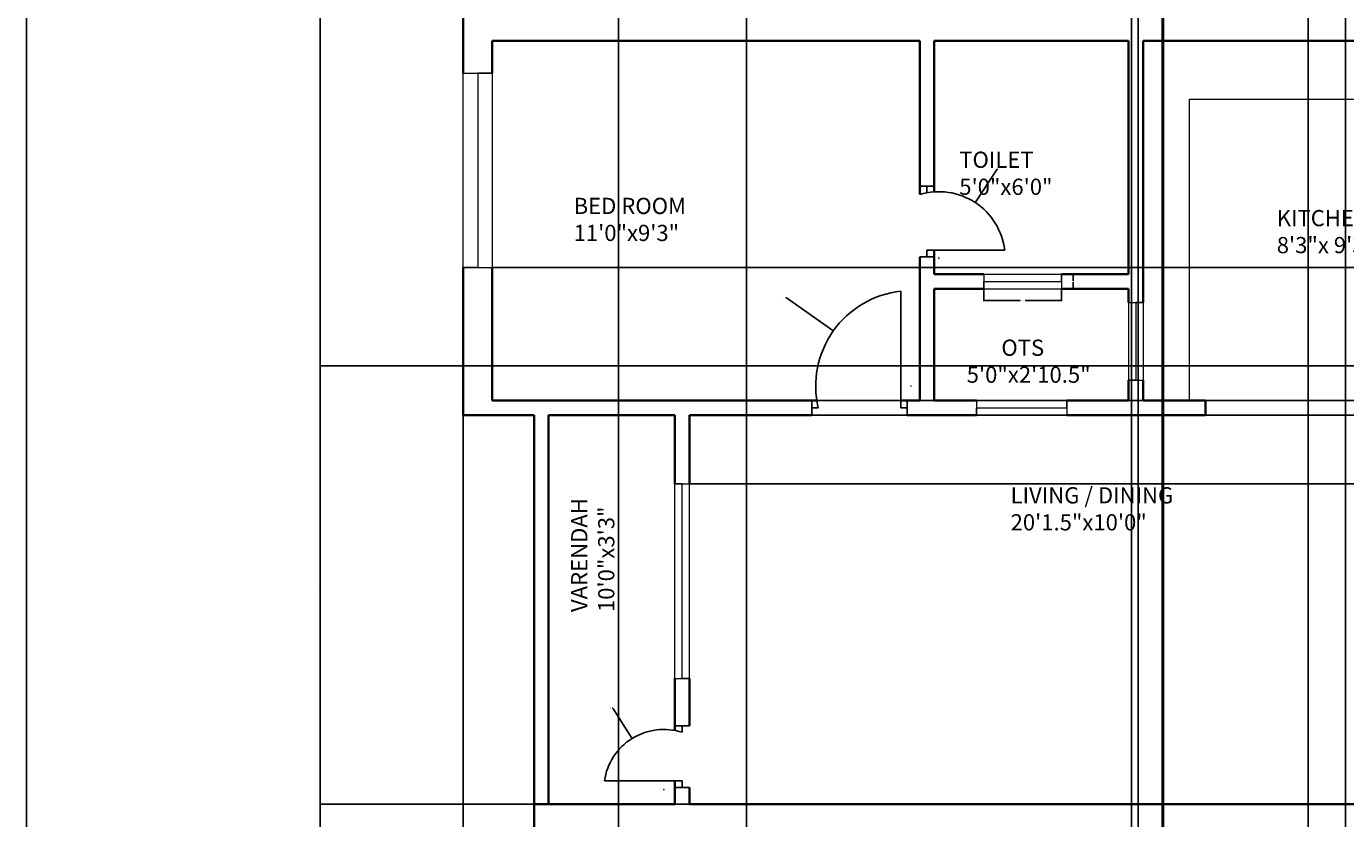
# Model space of a CAD drawing. Units: inches. Extents: x 1870 to 2611, y 1432 to 2511.
# Tile 3 of 5: x 1870 to 2277, y 1903 to 2147. Entities that reach past the tile are written whole.
import ezdxf

# ---------------------------------------------------------------- set-up
doc = ezdxf.new("R2010")
doc.units = ezdxf.units.IN
for name, color, linetype, lineweight in [('A-ANNO-DIMS', 2, 'Continuous', 18), ('A-ANNO-TTLB', 7, 'Continuous', 25), ('A-AREA-IDEN', 7, 'Continuous', 18), ('A-DOOR', 31, 'Continuous', 25), ('A-FLOR-FIXT', 8, 'Continuous', 18), ('A-GLAZ', 201, 'Continuous', 18), ('A-WALL', 7, 'Continuous', 35)]:
    doc.layers.add(name, color=color, linetype=linetype, lineweight=lineweight)
doc.styles.get("Standard").update_dxf_attribs({"font": 'arial.ttf'})
doc.dimstyles.get("Standard").update_dxf_attribs({"dimtxt": 0.18, "dimasz": 0.18, "dimexe": 0.18, "dimexo": 0.0625, "dimgap": 0.09, "dimtad": 0, "dimtih": 1, "dimtoh": 1, "dimdec": 4, "dimzin": 0, "dimdsep": 46, "dimtxsty": 'Standard', "dimcen": 0.09, "dimadec": 0, "dimazin": 0, "dimtfac": 1, "dimtdec": 4, "dimtofl": 0, "dimtmove": 0, "dimatfit": 3, "dimfxl": 1, "dimtolj": 1, "dimtzin": 0, "dimarcsym": 0})

# ---------------------------------------------------------------- blocks, each defined once
blk = doc.blocks.new('DOOR-LEAF-36-JAMB-4P5')
for p, q in [((36, 2), (0, 2)), ((33.75, 0), (38.25, 0)), ((36, 0), (36, 2)), ((38.25, 0), (36, 0))]:
    blk.add_line(p, q)
blk = doc.blocks.new('DOOR-LEAF-24-JAMB-4P5')
for p, q in [((2, 2.25), (2, 26.25)), ((0, 4.5), (0, 0)), ((0, 0), (0, 2.25)), ((0, 2.25), (2, 2.25))]:
    blk.add_line(p, q)
blk = doc.blocks.new('WIN-60-FRAME-9')
for p, q in [((0, 9), (0, 0)), ((60, 9), (0, 9)), ((60, 4.5), (60, 9)), ((60, 9), (60, 0)), ((0, 0), (0, 4.5)), ((0, 4.5), (60, 4.5)), ((0, 0), (60, 0))]:
    blk.add_line(p, q)
blk = doc.blocks.new('WIN-24-FRAME-4P5')
for p, q in [((0, 4.5), (0, 0)), ((0, 4.5), (24, 4.5)), ((24, 2.25), (24, 4.5)), ((24, 4.5), (24, 0)), ((0, 0), (0, 2.25)), ((0, 2.25), (24, 2.25)), ((0, 0), (24, 0))]:
    blk.add_line(p, q)
blk = doc.blocks.new('WIN-60-FRAME-4P5')
for p, q in [((0, 60), (4.5, 60)), ((0, 60), (0, 0)), ((4.5, 60), (2.25, 60)), ((2.25, 60), (2.25, 0)), ((4.5, 60), (4.5, 0)), ((2.25, 0), (0, 0)), ((0, 0), (4.5, 0))]:
    blk.add_line(p, q)
blk = doc.blocks.new('*D23')
at = {"layer": 'A-ANNO-DIMS', "color": 0, "lineweight": -2, "transparency": 16777216}
for p, q in [((2165.45, 2066.3), (2165.45, 2062.59)), ((2189.45, 2066.3), (2189.45, 2062.59)), ((2165.63, 2062.77), (2176.7, 2062.77)), ((2189.27, 2062.77), (2178.21, 2062.77))]:
    blk.add_line(p, q, dxfattribs=at)
at = {"layer": 'A-ANNO-DIMS', "color": 0, "transparency": 16777216}
for points in [[(2165.63, 2062.8), (2165.63, 2062.74), (2165.45, 2062.77)], [(2189.27, 2062.8), (2189.27, 2062.74), (2189.45, 2062.77)]]:
    blk.add_solid(points, dxfattribs=at)
at = {"layer": 'Defpoints', "color": 0, "transparency": 16777216}
for p in [(2165.45, 2066.37), (2189.45, 2066.37), (2189.45, 2062.77)]:
    blk.add_point(p, dxfattribs=at)
at = {"layer": 'A-ANNO-DIMS', "color": 0, "transparency": 16777216, "insert": (2177.45, 2062.77), "char_height": 0.18, "attachment_point": 5}
blk.add_mtext('\\A1;W4 24 TYP.', dxfattribs=at)
blk = doc.blocks.new('*D24')
at = {"layer": 'A-ANNO-DIMS', "color": 0, "lineweight": -2, "transparency": 16777216}
for p, q in [((2189.51, 2070.87), (2193.23, 2070.87)), ((2193.05, 2070.69), (2193.05, 2068.8)), ((2189.51, 2066.37), (2193.23, 2066.37)), ((2193.05, 2066.55), (2193.05, 2068.44))]:
    blk.add_line(p, q, dxfattribs=at)
at = {"layer": 'A-ANNO-DIMS', "color": 0, "transparency": 16777216}
for points in [[(2193.02, 2070.69), (2193.08, 2070.69), (2193.05, 2070.87)], [(2193.02, 2066.55), (2193.08, 2066.55), (2193.05, 2066.37)]]:
    blk.add_solid(points, dxfattribs=at)
at = {"layer": 'Defpoints', "color": 0, "transparency": 16777216}
for p in [(2189.45, 2070.87), (2193.05, 2070.87), (2189.45, 2066.37)]:
    blk.add_point(p, dxfattribs=at)
at = {"layer": 'A-ANNO-DIMS', "color": 0, "transparency": 16777216, "insert": (2193.05, 2068.62), "char_height": 0.18, "attachment_point": 5}
blk.add_mtext('\\A1;5 TYP.', dxfattribs=at)
blk = doc.blocks.new('*D28')
at = {"layer": 'A-ANNO-DIMS', "color": 0, "lineweight": -2, "transparency": 16777216}
for p, q in [((2004.57, 2151.87), (1960.31, 2151.87)), ((1960.49, 2151.69), (1960.49, 2029.8)), ((1960.49, 1907.55), (1960.49, 2029.44)), ((2026.46, 1907.37), (1960.31, 1907.37))]:
    blk.add_line(p, q, dxfattribs=at)
at = {"layer": 'A-ANNO-DIMS', "color": 0, "transparency": 16777216}
for points in [[(1960.46, 2151.69), (1960.52, 2151.69), (1960.49, 2151.87)], [(1960.46, 1907.55), (1960.52, 1907.55), (1960.49, 1907.37)]]:
    blk.add_solid(points, dxfattribs=at)
at = {"layer": 'Defpoints', "color": 0, "transparency": 16777216}
for p in [(2004.64, 2151.87), (1960.49, 1907.37), (2026.52, 1907.37)]:
    blk.add_point(p, dxfattribs=at)
at = {"layer": 'A-ANNO-DIMS', "color": 0, "transparency": 16777216, "insert": (1960.49, 2029.62), "char_height": 0.18, "attachment_point": 5}
blk.add_mtext('\\A1;244.5', dxfattribs=at)
blk = doc.blocks.new('*D29')
at = {"layer": 'A-ANNO-DIMS', "color": 0, "lineweight": -2, "transparency": 16777216}
for p, q in [((2026.46, 1907.37), (1960.31, 1907.37)), ((1960.49, 1907.19), (1960.49, 1774.05)), ((1960.49, 1640.55), (1960.49, 1773.69)), ((2026.46, 1640.37), (1960.31, 1640.37))]:
    blk.add_line(p, q, dxfattribs=at)
at = {"layer": 'A-ANNO-DIMS', "color": 0, "transparency": 16777216}
for points in [[(1960.46, 1907.19), (1960.52, 1907.19), (1960.49, 1907.37)], [(1960.46, 1640.55), (1960.52, 1640.55), (1960.49, 1640.37)]]:
    blk.add_solid(points, dxfattribs=at)
at = {"layer": 'Defpoints', "color": 0, "transparency": 16777216}
for p in [(2026.52, 1907.37), (1960.49, 1640.37), (2026.52, 1640.37)]:
    blk.add_point(p, dxfattribs=at)
at = {"layer": 'A-ANNO-DIMS', "color": 0, "transparency": 16777216, "insert": (1960.49, 1773.87), "char_height": 0.18, "attachment_point": 5}
blk.add_mtext('\\A1;267', dxfattribs=at)
blk = doc.blocks.new('*D30')
at = {"layer": 'A-ANNO-DIMS', "color": 0, "lineweight": -2, "transparency": 16777216}
for p, q in [((2004.64, 2027.3), (2004.64, 1485.35)), ((2026.52, 2027.3), (2026.52, 1485.35)), ((2004.82, 1485.53), (2015.11, 1485.53)), ((2026.34, 1485.53), (2016.04, 1485.53))]:
    blk.add_line(p, q, dxfattribs=at)
at = {"layer": 'A-ANNO-DIMS', "color": 0, "transparency": 16777216}
for points in [[(2004.82, 1485.56), (2004.82, 1485.5), (2004.64, 1485.53)], [(2026.34, 1485.56), (2026.34, 1485.5), (2026.52, 1485.53)]]:
    blk.add_solid(points, dxfattribs=at)
at = {"layer": 'Defpoints', "color": 0, "transparency": 16777216}
for p in [(2004.64, 2027.37), (2026.52, 2027.37), (2026.52, 1485.53)]:
    blk.add_point(p, dxfattribs=at)
at = {"layer": 'A-ANNO-DIMS', "color": 0, "transparency": 16777216, "insert": (2015.58, 1485.53), "char_height": 0.18, "attachment_point": 5}
blk.add_mtext('\\A1;21.882', dxfattribs=at)
blk = doc.blocks.new('*D34')
at = {"layer": 'A-ANNO-DIMS', "color": 0, "lineweight": -2, "transparency": 16777216}
for p, q in [((2385.57, 2042.61), (1960.31, 2042.61)), ((1960.49, 2042.43), (1960.49, 1975.17)), ((1960.49, 1907.55), (1960.49, 1974.8)), ((2385.57, 1907.37), (1960.31, 1907.37))]:
    blk.add_line(p, q, dxfattribs=at)
at = {"layer": 'A-ANNO-DIMS', "color": 0, "transparency": 16777216}
for points in [[(1960.46, 2042.43), (1960.52, 2042.43), (1960.49, 2042.61)], [(1960.46, 1907.55), (1960.52, 1907.55), (1960.49, 1907.37)]]:
    blk.add_solid(points, dxfattribs=at)
at = {"layer": 'Defpoints', "color": 0, "transparency": 16777216}
for p in [(1960.49, 2042.61), (2385.64, 2042.61), (2385.64, 1907.37)]:
    blk.add_point(p, dxfattribs=at)
at = {"layer": 'A-ANNO-DIMS', "color": 0, "transparency": 16777216, "insert": (1960.49, 1974.99), "char_height": 0.18, "attachment_point": 5}
blk.add_mtext('\\A1;135.24', dxfattribs=at)
blk = doc.blocks.new('*D39')
at = {"layer": 'A-ANNO-DIMS', "color": 0, "lineweight": -2, "transparency": 16777216}
for p, q in [((2052.64, 2396.3), (2052.64, 1485.35)), ((2092.09, 2396.3), (2092.09, 1485.35)), ((2052.82, 1485.53), (2071.97, 1485.53)), ((2091.91, 1485.53), (2072.76, 1485.53))]:
    blk.add_line(p, q, dxfattribs=at)
at = {"layer": 'A-ANNO-DIMS', "color": 0, "transparency": 16777216}
for points in [[(2052.82, 1485.56), (2052.82, 1485.5), (2052.64, 1485.53)], [(2091.91, 1485.56), (2091.91, 1485.5), (2092.09, 1485.53)]]:
    blk.add_solid(points, dxfattribs=at)
at = {"layer": 'Defpoints', "color": 0, "transparency": 16777216}
for p in [(2052.64, 2396.37), (2092.09, 2396.37), (2092.09, 1485.53)]:
    blk.add_point(p, dxfattribs=at)
at = {"layer": 'A-ANNO-DIMS', "color": 0, "transparency": 16777216, "insert": (2072.36, 1485.53), "char_height": 0.18, "attachment_point": 5}
blk.add_mtext('\\A1;39.45', dxfattribs=at)
blk = doc.blocks.new('*D40')
at = {"layer": 'A-ANNO-DIMS', "color": 0, "lineweight": -2, "transparency": 16777216}
for p, q in [((2213.14, 2396.3), (2213.14, 1485.35)), ((2220.9, 2396.3), (2220.9, 1485.35)), ((2213.32, 1485.53), (2216.63, 1485.53)), ((2220.72, 1485.53), (2217.41, 1485.53))]:
    blk.add_line(p, q, dxfattribs=at)
at = {"layer": 'A-ANNO-DIMS', "color": 0, "transparency": 16777216}
for points in [[(2213.32, 1485.56), (2213.32, 1485.5), (2213.14, 1485.53)], [(2220.72, 1485.56), (2220.72, 1485.5), (2220.9, 1485.53)]]:
    blk.add_solid(points, dxfattribs=at)
at = {"layer": 'Defpoints', "color": 0, "transparency": 16777216}
for p in [(2213.14, 2396.37), (2220.9, 2396.37), (2220.9, 1485.53)]:
    blk.add_point(p, dxfattribs=at)
at = {"layer": 'A-ANNO-DIMS', "color": 0, "transparency": 16777216, "insert": (2217.02, 1485.53), "char_height": 0.18, "attachment_point": 5}
blk.add_mtext('\\A1;7.766', dxfattribs=at)
blk = doc.blocks.new('*D41')
at = {"layer": 'A-ANNO-DIMS', "color": 0, "lineweight": -2, "transparency": 16777216}
for p, q in [((2265.64, 2396.3), (2265.64, 1485.35)), ((2277.17, 2396.3), (2277.17, 1485.35)), ((2265.82, 1485.53), (2270.95, 1485.53)), ((2276.99, 1485.53), (2271.86, 1485.53))]:
    blk.add_line(p, q, dxfattribs=at)
at = {"layer": 'A-ANNO-DIMS', "color": 0, "transparency": 16777216}
for points in [[(2265.82, 1485.56), (2265.82, 1485.5), (2265.64, 1485.53)], [(2276.99, 1485.56), (2276.99, 1485.5), (2277.17, 1485.53)]]:
    blk.add_solid(points, dxfattribs=at)
at = {"layer": 'Defpoints', "color": 0, "transparency": 16777216}
for p in [(2265.64, 2396.37), (2277.17, 2396.37), (2277.17, 1485.53)]:
    blk.add_point(p, dxfattribs=at)
at = {"layer": 'A-ANNO-DIMS', "color": 0, "transparency": 16777216, "insert": (2271.4, 1485.53), "char_height": 0.18, "attachment_point": 5}
blk.add_mtext('\\A1;11.535', dxfattribs=at)
blk = doc.blocks.new('*D45')
at = {"layer": 'A-ANNO-DIMS', "color": 0, "lineweight": -2, "transparency": 16777216}
for p, q in [((2211.02, 1649.43), (2211.02, 2449.7)), ((2211.2, 2449.52), (2215.39, 2449.52)), ((2220.38, 2449.52), (2216.18, 2449.52)), ((2220.56, 1649.43), (2220.56, 2449.7))]:
    blk.add_line(p, q, dxfattribs=at)
at = {"layer": 'A-ANNO-DIMS', "color": 0, "transparency": 16777216}
for points in [[(2211.2, 2449.55), (2211.2, 2449.49), (2211.02, 2449.52)], [(2220.38, 2449.55), (2220.38, 2449.49), (2220.56, 2449.52)]]:
    blk.add_solid(points, dxfattribs=at)
at = {"layer": 'Defpoints', "color": 0, "transparency": 16777216}
for p in [(2220.56, 2449.52), (2211.02, 1649.37), (2220.56, 1649.37)]:
    blk.add_point(p, dxfattribs=at)
at = {"layer": 'A-ANNO-DIMS', "color": 0, "transparency": 16777216, "insert": (2215.79, 2449.52), "char_height": 0.18, "attachment_point": 5}
blk.add_mtext('\\A1;9.537', dxfattribs=at)
blk = doc.blocks.new('*D51')
at = {"layer": 'A-ANNO-DIMS', "color": 0, "lineweight": -2, "transparency": 16777216}
for p, q in [((2013.7, 2072.92), (2524.47, 2072.92)), ((2524.29, 2072.74), (2524.29, 2052.57)), ((2524.29, 2032.05), (2524.29, 2052.21)), ((2013.7, 2031.87), (2524.47, 2031.87))]:
    blk.add_line(p, q, dxfattribs=at)
at = {"layer": 'A-ANNO-DIMS', "color": 0, "transparency": 16777216}
for points in [[(2524.26, 2072.74), (2524.32, 2072.74), (2524.29, 2072.92)], [(2524.26, 2032.05), (2524.32, 2032.05), (2524.29, 2031.87)]]:
    blk.add_solid(points, dxfattribs=at)
at = {"layer": 'Defpoints', "color": 0, "transparency": 16777216}
for p in [(2013.64, 2072.92), (2524.29, 2072.92), (2013.64, 2031.87)]:
    blk.add_point(p, dxfattribs=at)
at = {"layer": 'A-ANNO-DIMS', "color": 0, "transparency": 16777216, "insert": (2524.29, 2052.39), "char_height": 0.18, "attachment_point": 5}
blk.add_mtext('\\A1;41.05', dxfattribs=at)
blk = doc.blocks.new('*D54')
at = {"layer": 'A-ANNO-DIMS', "color": 0, "lineweight": -2, "transparency": 16777216}
for p, q in [((2074.58, 2027.37), (2524.47, 2027.37)), ((2524.29, 2027.19), (2524.29, 2016.94)), ((2524.29, 2006.33), (2524.29, 2016.58)), ((2074.58, 2006.15), (2524.47, 2006.15))]:
    blk.add_line(p, q, dxfattribs=at)
at = {"layer": 'A-ANNO-DIMS', "color": 0, "transparency": 16777216}
for points in [[(2524.26, 2027.19), (2524.32, 2027.19), (2524.29, 2027.37)], [(2524.26, 2006.33), (2524.32, 2006.33), (2524.29, 2006.15)]]:
    blk.add_solid(points, dxfattribs=at)
at = {"layer": 'Defpoints', "color": 0, "transparency": 16777216}
for p in [(2074.52, 2027.37), (2524.29, 2027.37), (2074.52, 2006.15)]:
    blk.add_point(p, dxfattribs=at)
at = {"layer": 'A-ANNO-DIMS', "color": 0, "transparency": 16777216, "insert": (2524.29, 2016.76), "char_height": 0.18, "attachment_point": 5}
blk.add_mtext('\\A1;21.215', dxfattribs=at)
blk = doc.blocks.new('*D61')
at = {"layer": 'A-ANNO-DIMS', "color": 0, "lineweight": -2, "transparency": 16777216}
for p, q in [((2104.34, 2063.56), (2104.52, 2063.56)), ((2104.52, 2063.56), (2118.78, 2053.47)), ((2142.85, 2036.37), (2143.03, 2036.37)), ((2142.94, 2036.28), (2142.94, 2036.46))]:
    blk.add_line(p, q, dxfattribs=at)
at = {"layer": 'A-ANNO-DIMS', "color": 0, "transparency": 16777216}
blk.add_solid([(2118.8, 2053.49), (2118.76, 2053.44), (2118.93, 2053.36)], dxfattribs=at)
at = {"layer": 'Defpoints', "color": 0, "transparency": 16777216}
for p in [(2118.93, 2053.36), (2142.94, 2036.37)]:
    blk.add_point(p, dxfattribs=at)
at = {"layer": 'A-ANNO-DIMS', "color": 0, "transparency": 16777216, "insert": (2103.86, 2063.56), "char_height": 0.18, "attachment_point": 5}
blk.add_mtext('\\A1;R29.42', dxfattribs=at)
blk = doc.blocks.new('*D69')
at = {"layer": 'A-ANNO-DIMS', "color": 0, "lineweight": -2, "transparency": 16777216}
for p, q in [((2169.52, 2103.29), (2162.86, 2093.15)), ((2169.7, 2103.29), (2169.52, 2103.29)), ((2151.42, 2075.84), (2151.6, 2075.84)), ((2151.51, 2075.75), (2151.51, 2075.93))]:
    blk.add_line(p, q, dxfattribs=at)
at = {"layer": 'A-ANNO-DIMS', "color": 0, "transparency": 16777216}
blk.add_solid([(2162.84, 2093.16), (2162.89, 2093.13), (2162.76, 2093)], dxfattribs=at)
at = {"layer": 'Defpoints', "color": 0, "transparency": 16777216}
for p in [(2162.76, 2093), (2151.51, 2075.84)]:
    blk.add_point(p, dxfattribs=at)
at = {"layer": 'A-ANNO-DIMS', "color": 0, "transparency": 16777216, "insert": (2170.17, 2103.29), "char_height": 0.18, "attachment_point": 5}
blk.add_mtext('\\A1;R20.52', dxfattribs=at)
blk = doc.blocks.new('*D73')
at = {"layer": 'A-ANNO-DIMS', "color": 0, "lineweight": -2, "transparency": 16777216}
for p, q in [((2050.73, 1937), (2050.91, 1937)), ((2050.91, 1937), (2056.69, 1927.73)), ((2066.5, 1911.89), (2066.68, 1911.89)), ((2066.59, 1911.8), (2066.59, 1911.98))]:
    blk.add_line(p, q, dxfattribs=at)
at = {"layer": 'A-ANNO-DIMS', "color": 0, "transparency": 16777216}
blk.add_solid([(2056.72, 1927.75), (2056.67, 1927.72), (2056.79, 1927.58)], dxfattribs=at)
at = {"layer": 'Defpoints', "color": 0, "transparency": 16777216}
for p in [(2056.79, 1927.58), (2066.59, 1911.89)]:
    blk.add_point(p, dxfattribs=at)
at = {"layer": 'A-ANNO-DIMS', "color": 0, "transparency": 16777216, "insert": (2050.32, 1937), "char_height": 0.18, "attachment_point": 5}
blk.add_mtext('\\A1;R18.5', dxfattribs=at)

msp = doc.modelspace()

# ---------------------------------------------------------------- linework, layer by layer
at = {"layer": 'A-ANNO-TTLB'}
msp.add_lwpolyline([(1869.7418, 2510.8018), (2611.0646, 2510.8018), (2611.0646, 1431.531), (1869.7418, 1431.531)], close=True, dxfattribs=at)
at = {"layer": 'A-DOOR'}
for p, q in [((2145.6359, 2098.0357), (2150.1359, 2098.0357)), ((2150.1359, 2098.0357), (2147.8859, 2098.0357)), ((2147.8859, 2098.0357), (2147.8859, 2096.0357)), ((2145.6359, 2076.2857), (2145.6359, 2076.2857)), ((2145.6359, 2076.2857), (2150.1359, 2076.2857)), ((2112.3075, 2031.8669), (2112.3075, 2027.3669)), ((2112.3075, 2027.3669), (2112.3075, 2029.6169)), ((2112.3075, 2029.6169), (2114.3075, 2029.6169)), ((2070.0182, 1931.4958), (2074.5182, 1931.4958)), ((2074.5182, 1931.4958), (2072.2682, 1931.4958)), ((2072.2682, 1931.4958), (2072.2682, 1929.4958)), ((2072.2746, 1914.5136), (2048.2746, 1914.5136)), ((2070.0182, 1912.5136), (2070.0182, 1912.5136)), ((2070.0182, 1912.5136), (2073.3159, 1912.5136)), ((2072.2746, 1912.5136), (2072.2746, 1914.5136)), ((2074.5182, 1912.5136), (2072.2746, 1912.5136)), ((2073.3159, 1912.5136), (2074.5182, 1912.5136))]:
    msp.add_line(p, q, dxfattribs=at)
for centre, radius, start, end in [((2151.5111, 2075.8369), 20.5215, 6.853149, 106.636068), ((2142.9403, 2036.3683), 29.4181, 96.152009, 193.267453), ((2066.5868, 1911.8907), 18.4991, 72.114348, 171.848928)]:
    msp.add_arc(centre, radius, start, end, dxfattribs=at)
at = {"layer": 'A-FLOR-FIXT'}
for p, q in [((2228.9306, 2031.8669), (2228.9306, 2124.8754)), ((2228.9306, 2124.8754), (2313.6359, 2124.8754))]:
    msp.add_line(p, q, dxfattribs=at)
at = {"layer": 'A-GLAZ'}
for p, q in [((2013.6359, 2072.9155), (2013.6359, 2072.9155)), ((2210.1359, 2062.1962), (2210.1359, 2062.1962)), ((2163.1231, 2031.8669), (2163.1231, 2027.3669)), ((2163.1231, 2027.3669), (2163.1231, 2029.6169)), ((2163.1231, 2029.6169), (2191.0748, 2029.6169)), ((2191.0748, 2029.6169), (2191.0748, 2031.8669)), ((2191.0748, 2031.8669), (2191.0748, 2027.3669))]:
    msp.add_line(p, q, dxfattribs=at)
at = {"layer": 'A-WALL'}
for p, q in [((2004.6359, 2405.3669), (2004.6359, 2132.9155)), ((2013.6359, 2142.8669), (2145.6359, 2142.8669)), ((2013.6359, 2142.8669), (2013.6359, 2132.9155)), ((2145.6359, 2095.4995), (2145.6359, 2142.8669)), ((2150.1359, 2142.8669), (2150.1359, 2096.3123)), ((2150.1359, 2142.8669), (2210.1359, 2142.8669)), ((2150.1359, 2142.8669), (2150.1359, 2096.3123)), ((2210.1359, 2142.8669), (2210.1359, 2142.8669)), ((2210.1359, 2070.8669), (2210.1359, 2142.8669)), ((2214.6359, 2142.8669), (2214.6359, 2062.1962)), ((2214.6359, 2142.8669), (2313.6359, 2142.8669)), ((2150.1359, 2078.2857), (2150.1359, 2070.8669)), ((2150.1359, 2078.2857), (2150.1359, 2070.8669)), ((2145.6359, 2031.8669), (2145.6359, 2076.2857)), ((2004.6359, 2072.9155), (2004.6359, 2027.3669)), ((2013.6359, 2072.9155), (2013.6359, 2031.8669)), ((2150.1359, 2070.8669), (2165.4524, 2070.8669)), ((2189.4524, 2070.8669), (2210.1359, 2070.8669)), ((2210.1359, 2070.8669), (2210.1359, 2070.8669)), ((2150.1359, 2066.3669), (2150.1359, 2031.8669)), ((2165.4524, 2066.3669), (2150.1359, 2066.3669)), ((2210.1359, 2066.3669), (2189.4524, 2066.3669)), ((2210.1359, 2062.1962), (2210.1359, 2066.3669)), ((2210.1359, 2031.8669), (2210.1359, 2038.1962)), ((2214.6359, 2038.1962), (2214.6359, 2031.8669)), ((2013.6359, 2031.8669), (2113.8687, 2031.8669)), ((2013.6359, 2031.8669), (2113.8687, 2031.8669)), ((2139.7877, 2031.8669), (2145.6359, 2031.8669)), ((2139.7877, 2031.8669), (2145.6359, 2031.8669)), ((2150.1359, 2031.8669), (2163.1231, 2031.8669)), ((2150.1359, 2031.8669), (2163.1231, 2031.8669)), ((2191.0748, 2031.8669), (2210.1359, 2031.8669)), ((2191.0748, 2031.8669), (2210.1359, 2031.8669)), ((2214.6359, 2031.8669), (2233.9327, 2031.8669)), ((2214.6359, 2031.8669), (2233.9327, 2031.8669)), ((2233.9327, 2031.8669), (2233.9327, 2027.3669)), ((2004.6359, 2027.3669), (2026.5182, 2027.3669)), ((2026.5182, 2027.3669), (2026.5182, 1640.3669)), ((2031.0182, 2027.3669), (2031.0182, 1907.3669)), ((2031.0182, 2027.3669), (2048.1359, 2027.3669)), ((2052.6359, 2027.3669), (2048.1359, 2027.3669)), ((2052.6359, 2027.3669), (2070.0182, 2027.3669)), ((2070.0182, 2027.3669), (2070.0182, 2006.1522)), ((2074.5182, 2027.3669), (2074.5182, 2006.1522)), ((2074.5182, 2027.3669), (2112.3075, 2027.3669)), ((2141.7877, 2027.3669), (2163.1231, 2027.3669)), ((2191.0748, 2027.3669), (2233.9327, 2027.3669)), ((2070.0182, 1946.1522), (2070.0182, 1930.0688)), ((2074.5182, 1946.1522), (2074.5182, 1931.4958)), ((2070.0182, 1914.5136), (2070.0182, 1907.3669)), ((2074.5182, 1912.5136), (2074.5182, 1907.3669)), ((2026.5182, 1907.3669), (2070.0182, 1907.3669)), ((2074.5182, 1907.3669), (2313.6359, 1907.3669))]:
    msp.add_line(p, q, dxfattribs=at)

# ---------------------------------------------------------------- block references
at = {"layer": 'A-DOOR', "extrusion": (0, 0, -1), "zscale": -1}
for name, p, rotation in [('DOOR-LEAF-24-JAMB-4P5', (-2145.636, 2076.2854), 89.99999999999991), ('DOOR-LEAF-36-JAMB-4P5', (-2141.7878, 2065.6169), 270.0000000000008)]:
    msp.add_blockref(name, p, dxfattribs=dict(at, rotation=rotation))
at = {"layer": 'A-GLAZ', "extrusion": (0, 0, -1), "zscale": -1}
for name, p, rotation in [('WIN-60-FRAME-9', (-2013.6359, 2132.9153), 269.9999999999999), ('WIN-24-FRAME-4P5', (-2214.6359, 2062.1966), 270.0000000000035), ('WIN-60-FRAME-4P5', (-2070.0183, 2006.1521), 180)]:
    msp.add_blockref(name, p, dxfattribs=dict(at, rotation=rotation))
at = {"layer": 'A-GLAZ'}
msp.add_blockref('WIN-24-FRAME-4P5', (2165.452, 2066.367), dxfattribs=at)

# ---------------------------------------------------------------- texts
at = {"layer": 'A-AREA-IDEN', "char_height": 5, "attachment_point": 1}
for s, width, insert in [('TOILET\\P5\'0"x6\'0"', 56.787286, (2157.8486, 2108.7055)), ('BED ROOM\\P11\'0"x9\'3"', 133.560521, (2038.7525, 2094.4601)), ('KITCHEN\\P8\'3"x 9\'3"', 77.76941, (2255.9057, 2090.7047)), ('       OTS\\P5\'0"x2\'10.5"', 43.4584, (2160.1509, 2050.7093)), ('LIVING / DINING\\P20\'1.5"x10\'0"', 75.50488, (2173.7033, 2005.1462))]:
    msp.add_mtext_dynamic_manual_height_columns(s, width=width, gutter_width=12.5, heights=[0], dxfattribs=dict(at, insert=insert))
at = {"layer": 'A-AREA-IDEN', "insert": (2037.9898, 1966.6105), "char_height": 5, "attachment_point": 1, "rotation": 90}
msp.add_mtext_dynamic_manual_height_columns('VARENDAH\\P10\'0"x3\'3" ', width=67.65528, gutter_width=12.5, heights=[0], dxfattribs=at)

# ---------------------------------------------------------------- dimensions: what is measured, and where the dimension line sits
at = {"layer": 'A-ANNO-DIMS'}
for base, p1, p2, override, picture, middle in [((2220.55567, 2449.51694), (2211.01824, 1649.36694), (2220.55567, 1649.36694), {"dimdec": 3, "dimlfac": 1, "dimrnd": 0, "dimzin": 0, "dimdsep": 46, "dimlunit": 2}, '*D45', (2215.78695, 2449.51694)), ((2092.0868, 1485.5313), (2052.6359, 2396.3669), (2092.0868, 2396.3669), {"dimdec": 2, "dimlfac": 1, "dimrnd": 0, "dimzin": 0, "dimdsep": 46, "dimlunit": 2}, '*D39', (2072.3614, 1485.5313)), ((2220.9018, 1485.5313), (2213.1359, 2396.3669), (2220.9018, 2396.3669), {"dimdec": 3, "dimlfac": 1, "dimrnd": 0, "dimzin": 0, "dimdsep": 46, "dimlunit": 2}, '*D40', (2217.0189, 1485.5313)), ((2277.1709, 1485.5313), (2265.6359, 2396.3669), (2277.1709, 2396.3669), {"dimdec": 3, "dimlfac": 1, "dimrnd": 0, "dimzin": 0, "dimdsep": 46, "dimlunit": 2}, '*D41', (2271.4034, 1485.5313)), ((2026.5182, 1485.5313), (2004.6359, 2027.3669), (2026.5182, 2027.3669), {"dimdec": 3, "dimlfac": 1, "dimrnd": 0, "dimzin": 0, "dimdsep": 46, "dimlunit": 2}, '*D30', (2015.5771, 1485.5313))]:
    dim = msp.add_linear_dim(base=base, p1=p1, p2=p2, dimstyle='Standard', override=override, dxfattribs=at)
    dim.commit()
    dim.dimension.update_dxf_attribs({"geometry": picture, "text_midpoint": middle})
for base, p1, p2, override, picture, middle in [((1960.4859, 1907.3669), (2004.6359, 2151.8669), (2026.5182, 1907.3669), {"dimdec": 1, "dimlfac": 1, "dimrnd": 0, "dimzin": 0, "dimdsep": 46, "dimlunit": 2}, '*D28', (1960.4859, 2029.6169)), ((2524.2859, 2072.9155), (2013.6359, 2031.8669), (2013.6359, 2072.9155), {"dimdec": 2, "dimlfac": 1, "dimrnd": 0, "dimzin": 0, "dimdsep": 46, "dimlunit": 2}, '*D51', (2524.2859, 2052.3912)), ((1960.4859, 2042.6068), (2385.6359, 1907.3669), (2385.6359, 2042.6068), {"dimdec": 2, "dimlfac": 1, "dimrnd": 0, "dimzin": 0, "dimdsep": 46, "dimlunit": 2}, '*D34', (1960.4859, 1974.9869)), ((2524.2859, 2027.3669), (2074.5182, 2006.1522), (2074.5182, 2027.3669), {"dimdec": 3, "dimlfac": 1, "dimrnd": 0, "dimzin": 0, "dimdsep": 46, "dimlunit": 2}, '*D54', (2524.2859, 2016.7595)), ((1960.4859, 1640.3669), (2026.5182, 1907.3669), (2026.5182, 1640.3669), {"dimdec": 0, "dimlfac": 1, "dimrnd": 0, "dimzin": 0, "dimdsep": 46, "dimlunit": 2}, '*D29', (1960.4859, 1773.8669))]:
    dim = msp.add_linear_dim(base=base, p1=p1, p2=p2, angle=90, dimstyle='Standard', override=override, dxfattribs=at)
    dim.commit()
    dim.dimension.update_dxf_attribs({"geometry": picture, "text_midpoint": middle})
for center, mpoint, override, picture, middle in [((2151.5111, 2075.8369), (2162.764, 2092.998), {"dimdec": 2, "dimlfac": 1, "dimrnd": 0, "dimzin": 0, "dimdsep": 46, "dimlunit": 2}, '*D69', (2170.1747, 2103.2947)), ((2142.9403, 2036.3683), (2118.9283, 2053.3638), {"dimdec": 2, "dimlfac": 1, "dimrnd": 0, "dimzin": 0, "dimdsep": 46, "dimlunit": 2}, '*D61', (2103.8622, 2063.5611)), ((2066.5868, 1911.8907), (2056.7889, 1927.5821), {"dimdec": 1, "dimlfac": 1, "dimrnd": 0, "dimzin": 0, "dimdsep": 46, "dimlunit": 2}, '*D73', (2050.3196, 1936.9969))]:
    dim = msp.add_radius_dim(center=center, mpoint=mpoint, dimstyle='Standard', override=override, dxfattribs=at)
    dim.commit()
    dim.dimension.update_dxf_attribs({"geometry": picture, "text_midpoint": middle, "dimtype": 164})
dim = msp.add_linear_dim(base=(2193.0523992756, 2070.8669377198), p1=(2189.4523992756, 2066.3669377198), p2=(2189.4523992756, 2070.8669377198), angle=90, text='<> TYP.', dimstyle='Standard', override={"dimdec": 0, "dimlfac": 1, "dimrnd": 0, "dimzin": 0, "dimdsep": 46, "dimlunit": 2}, dxfattribs=at)
dim.commit()
dim.dimension.update_dxf_attribs({"geometry": '*D24', "text_midpoint": (2193.0523992756, 2068.6169377198)})
dim = msp.add_linear_dim(base=(2189.4524, 2062.7669), p1=(2165.4524, 2066.3669), p2=(2189.4524, 2066.3669), text='W4 <> TYP.', dimstyle='Standard', override={"dimdec": 0, "dimlfac": 1, "dimrnd": 0, "dimzin": 0, "dimdsep": 46, "dimlunit": 2}, dxfattribs=at)
dim.commit()
dim.dimension.update_dxf_attribs({"geometry": '*D23', "text_midpoint": (2177.4524, 2062.7669)})

doc.saveas('drawing.dxf')
